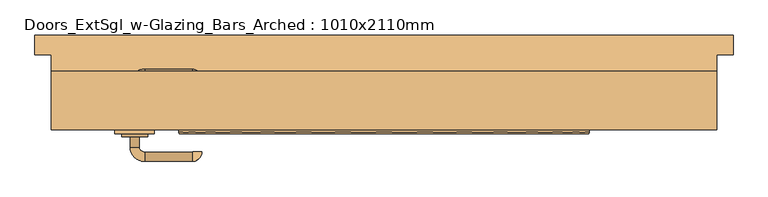
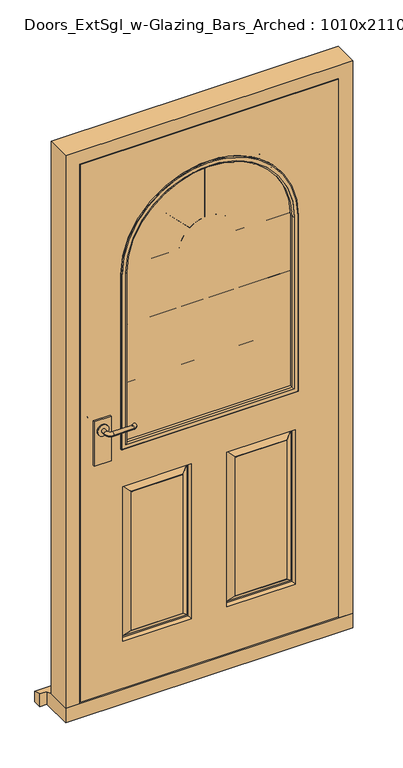
"""IFC4 building model written with IfcOpenShell, lengths in millimetres: door geometry, Doors_ExtSgl_w-Glazing_Bars_Arched : 1010x2110mm."""

from ifc_helpers import new_model, si_unit, point, frame, frame_2d, origin, place, context, project, spatial, polyline, circle_curve, ellipse_curve, trimmed, segment, composite_curve, outline, extrude, faceted_brep, source, transform, mapped, element, save
from ifc_brep_helpers import plane_surface, cylinder_surface, revolved_surface, advanced_brep


def doors_extsgl_w_glazing_bars_arched_1010x2110mm_bccdb1b2(model_context):
    return source(origin(), model_context, "Body", "SolidModel", [
        extrude(outline(composite_curve([segment(trimmed(circle_curve(frame_2d((1050.0, -378.5)), 20.0), [point((1050.0, -398.5))], [point((1050.0, -358.5))], False, "CARTESIAN"), True, "CONTINUOUS"), segment(trimmed(circle_curve(frame_2d((1050.0, -378.5)), 20.0), [point((1050.0, -358.5))], [point((1050.0, -398.5))], False, "CARTESIAN"), True, "CONTINUOUS")], self_intersect=False)), frame((0.0, -22.9929895, 0.0), z_axis=(0.0, 1.0, 0.0), x_axis=(0.0, 0.0, 1.0)), (0.0, 0.0, 1.0), 4.5929895),
        advanced_brep(
        [(-371.5, -22.9929895, 1050.0), (-385.5, -22.9929895, 1050.0), (-385.5, -38.4, 1050.0), (-371.5, -38.4, 1050.0), (-363.5, -60.4, 1050.0), (-363.5, -46.4, 1050.0), (-291.5, -60.4, 1050.0), (-291.5, -46.4, 1050.0), (-290.5, -45.4, 1050.0), (-276.5, -45.4, 1050.0)],
        [
            (0, 1, circle_curve(frame((-378.5, -22.9929895, 1050.0), z_axis=(0.0, 1.0, 0.0), x_axis=(-1.0, 0.0, 0.0)), 7.0)),
            (1, 0, circle_curve(frame((-378.5, -22.9929895, 1050.0), z_axis=(0.0, 1.0, 0.0), x_axis=(-1.0, 0.0, 0.0)), 7.0)),
            (1, 2),
            (2, 3, circle_curve(frame((-378.5, -38.4, 1050.0), z_axis=(0.0, 1.0, 0.0), x_axis=(-1.0, 0.0, 0.0)), 7.0)),
            (3, 0),
            (3, 2, circle_curve(frame((-378.5, -38.4, 1050.0), z_axis=(0.0, 1.0, 0.0), x_axis=(-1.0, 0.0, 0.0)), 7.0)),
            (4, 5, circle_curve(frame((-363.5, -53.4, 1050.0), z_axis=(-1.0, 0.0, 0.0), x_axis=(0.0, -1.0, 0.0)), 7.0)),
            (5, 3, circle_curve(frame((-363.5, -38.4, 1050.0), z_axis=(0.0, 0.0, -1.0), x_axis=(-1.0, 0.0, 0.0)), 8.0)),
            (2, 4, circle_curve(frame((-363.5, -38.4, 1050.0), z_axis=(0.0, 0.0, 1.0), x_axis=(-1.0, 0.0, 0.0)), 22.0)),
            (5, 4, circle_curve(frame((-363.5, -53.4, 1050.0), z_axis=(-1.0, 0.0, 0.0), x_axis=(0.0, -1.0, 0.0)), 7.0)),
            (4, 6),
            (6, 7, circle_curve(frame((-291.5, -53.4, 1050.0), z_axis=(-1.0, 0.0, 0.0), x_axis=(0.0, -1.0, 0.0)), 7.0)),
            (7, 5),
            (7, 6, circle_curve(frame((-291.5, -53.4, 1050.0), z_axis=(-1.0, 0.0, 0.0), x_axis=(0.0, -1.0, 0.0)), 7.0)),
            (8, 9, circle_curve(frame((-283.5, -45.4, 1050.0), z_axis=(0.0, 1.0, 0.0), x_axis=(1.0, 0.0, 0.0)), 7.0)),
            (9, 8, circle_curve(frame((-283.5, -45.4, 1050.0), z_axis=(0.0, 1.0, 0.0), x_axis=(1.0, 0.0, 0.0)), 7.0)),
            (8, 7, circle_curve(frame((-291.5, -45.4, 1050.0), z_axis=(0.0, 0.0, -1.0), x_axis=(0.0, -1.0, 0.0)), 1.0)),
            (6, 9, circle_curve(frame((-291.5, -45.4, 1050.0), z_axis=(0.0, 0.0, 1.0), x_axis=(0.0, -1.0, 0.0)), 15.0)),
        ],
        [
            plane_surface(frame((-378.5, -22.9929895, 1050.0), z_axis=(0.0, 1.0, 0.0), x_axis=(0.0, 0.0, 1.0))),
            cylinder_surface(frame((-378.5, -22.9929895, 1050.0), z_axis=(0.0, 1.0, 0.0), x_axis=(-1.0, 0.0, 0.0)), 7.0),
            revolved_surface(trimmed(ellipse_curve(frame((-378.5, -38.4, 1050.0), z_axis=(0.0, -1.0, 0.0), x_axis=(-1.0, 0.0, 0.0)), 7.0, 7.0), [point((-371.5, -38.4, 1050.0))], [point((-385.5, -38.4, 1050.0))], True, "CARTESIAN"), (-363.5, -38.4, 1050.0), (0.0, 0.0, -1.0)),
            revolved_surface(trimmed(ellipse_curve(frame((-378.5, -38.4, 1050.0), z_axis=(0.0, -1.0, 0.0), x_axis=(-1.0, 0.0, 0.0)), 7.0, 7.0), [point((-385.5, -38.4, 1050.0))], [point((-371.5, -38.4, 1050.0))], True, "CARTESIAN"), (-363.5, -38.4, 1050.0), (0.0, 0.0, -1.0)),
            cylinder_surface(frame((-363.5, -53.4, 1050.0), z_axis=(-1.0, 0.0, 0.0), x_axis=(0.0, -1.0, 0.0)), 7.0),
            plane_surface(frame((-283.5, -45.4, 1050.0), z_axis=(0.0, 1.0, 0.0), x_axis=(0.0, 0.0, 1.0))),
            revolved_surface(trimmed(ellipse_curve(frame((-291.5, -53.4, 1050.0), z_axis=(1.0, 0.0, 0.0), x_axis=(0.0, -1.0, 0.0)), 7.0, 7.0), [point((-291.5, -46.4, 1050.0))], [point((-291.5, -60.4, 1050.0))], True, "CARTESIAN"), (-291.5, -45.4, 1050.0), (0.0, 0.0, -1.0)),
            revolved_surface(trimmed(ellipse_curve(frame((-291.5, -53.4, 1050.0), z_axis=(1.0, 0.0, 0.0), x_axis=(0.0, -1.0, 0.0)), 7.0, 7.0), [point((-291.5, -60.4, 1050.0))], [point((-291.5, -46.4, 1050.0))], True, "CARTESIAN"), (-291.5, -45.4, 1050.0), (0.0, 0.0, -1.0)),
        ],
        [
            (0, [[1, 2]]),
            (1, [[3, 4, 5, -2]]),
            (1, [[-5, 6, -3, -1]]),
            (2, [[7, 8, -4, 9]]),
            (3, [[10, -9, -6, -8]]),
            (4, [[11, 12, 13, -7]]),
            (4, [[-13, 14, -11, -10]]),
            (5, [[15, 16]]),
            (6, [[-15, 17, -12, 18]]),
            (7, [[-16, -18, -14, -17]]),
        ],
    ),
        extrude(outline(polyline([(-348.5, -12.4), (-348.5, -18.4), (-408.5, -18.4), (-408.5, -12.4), (-348.5, -12.4)])), frame((0.0, 0.0, 925.0), z_axis=(0.0, 0.0, 1.0), x_axis=(1.0, 0.0, 0.0)), (0.0, 0.0, 1.0), 165.0),
        extrude(outline(composite_curve([segment(trimmed(circle_curve(frame_2d((1050.0, -378.5)), 20.0), [point((1050.0, -398.5))], [point((1050.0, -358.5))], False, "CARTESIAN"), True, "CONTINUOUS"), segment(trimmed(circle_curve(frame_2d((1050.0, -378.5)), 20.0), [point((1050.0, -358.5))], [point((1050.0, -398.5))], False, "CARTESIAN"), True, "CONTINUOUS")], self_intersect=False)), frame((0.0, 37.6, 0.0), z_axis=(0.0, 1.0, 0.0), x_axis=(0.0, 0.0, 1.0)), (0.0, 0.0, 1.0), 4.5929895),
        advanced_brep(
        [(-371.5, 42.1929895, 1050.0), (-385.5, 42.1929895, 1050.0), (-371.5, 57.6, 1050.0), (-385.5, 57.6, 1050.0), (-363.5, 79.6, 1050.0), (-363.5, 65.6, 1050.0), (-291.5, 65.6, 1050.0), (-291.5, 79.6, 1050.0), (-290.5, 64.6, 1050.0), (-276.5, 64.6, 1050.0)],
        [
            (0, 1, circle_curve(frame((-378.5, 42.1929895, 1050.0), z_axis=(0.0, -1.0, 0.0), x_axis=(-1.0, 0.0, 0.0)), 7.0)),
            (1, 0, circle_curve(frame((-378.5, 42.1929895, 1050.0), z_axis=(0.0, -1.0, 0.0), x_axis=(-1.0, 0.0, 0.0)), 7.0)),
            (0, 2),
            (2, 3, circle_curve(frame((-378.5, 57.6, 1050.0), z_axis=(0.0, -1.0, 0.0), x_axis=(-1.0, 0.0, 0.0)), 7.0)),
            (3, 1),
            (3, 2, circle_curve(frame((-378.5, 57.6, 1050.0), z_axis=(0.0, -1.0, 0.0), x_axis=(-1.0, 0.0, 0.0)), 7.0)),
            (4, 3, circle_curve(frame((-363.5, 57.6, 1050.0), z_axis=(0.0, 0.0, 1.0), x_axis=(-1.0, 0.0, 0.0)), 22.0)),
            (2, 5, circle_curve(frame((-363.5, 57.6, 1050.0), z_axis=(0.0, 0.0, -1.0), x_axis=(-1.0, 0.0, 0.0)), 8.0)),
            (5, 4, circle_curve(frame((-363.5, 72.6, 1050.0), z_axis=(-1.0, 0.0, 0.0), x_axis=(0.0, 1.0, 0.0)), 7.0)),
            (4, 5, circle_curve(frame((-363.5, 72.6, 1050.0), z_axis=(-1.0, 0.0, 0.0), x_axis=(0.0, 1.0, 0.0)), 7.0)),
            (5, 6),
            (6, 7, circle_curve(frame((-291.5, 72.6, 1050.0), z_axis=(-1.0, 0.0, 0.0), x_axis=(0.0, 1.0, 0.0)), 7.0)),
            (7, 4),
            (7, 6, circle_curve(frame((-291.5, 72.6, 1050.0), z_axis=(-1.0, 0.0, 0.0), x_axis=(0.0, 1.0, 0.0)), 7.0)),
            (8, 9, circle_curve(frame((-283.5, 64.6, 1050.0), z_axis=(0.0, -1.0, 0.0), x_axis=(1.0, 0.0, 0.0)), 7.0)),
            (9, 8, circle_curve(frame((-283.5, 64.6, 1050.0), z_axis=(0.0, -1.0, 0.0), x_axis=(1.0, 0.0, 0.0)), 7.0)),
            (9, 7, circle_curve(frame((-291.5, 64.6, 1050.0), z_axis=(0.0, 0.0, 1.0), x_axis=(0.0, 1.0, 0.0)), 15.0)),
            (6, 8, circle_curve(frame((-291.5, 64.6, 1050.0), z_axis=(0.0, 0.0, -1.0), x_axis=(0.0, 1.0, 0.0)), 1.0)),
        ],
        [
            plane_surface(frame((-378.5, 42.1929895, 1050.0), z_axis=(0.0, -1.0, 0.0), x_axis=(0.0, 0.0, 1.0))),
            cylinder_surface(frame((-378.5, 42.1929895, 1050.0), z_axis=(0.0, -1.0, 0.0), x_axis=(-1.0, 0.0, 0.0)), 7.0),
            revolved_surface(trimmed(ellipse_curve(frame((-378.5, 57.6, 1050.0), z_axis=(0.0, -1.0, 0.0), x_axis=(-1.0, 0.0, 0.0)), 7.0, 7.0), [point((-371.5, 57.6, 1050.0))], [point((-385.5, 57.6, 1050.0))], True, "CARTESIAN"), (-363.5, 57.6, 1050.0), (0.0, 0.0, -1.0)),
            revolved_surface(trimmed(ellipse_curve(frame((-378.5, 57.6, 1050.0), z_axis=(0.0, -1.0, 0.0), x_axis=(-1.0, 0.0, 0.0)), 7.0, 7.0), [point((-385.5, 57.6, 1050.0))], [point((-371.5, 57.6, 1050.0))], True, "CARTESIAN"), (-363.5, 57.6, 1050.0), (0.0, 0.0, -1.0)),
            cylinder_surface(frame((-363.5, 72.6, 1050.0), z_axis=(-1.0, 0.0, 0.0), x_axis=(0.0, 1.0, 0.0)), 7.0),
            plane_surface(frame((-283.5, 64.6, 1050.0), z_axis=(0.0, -1.0, 0.0), x_axis=(0.0, 0.0, 1.0))),
            revolved_surface(trimmed(ellipse_curve(frame((-291.5, 72.6, 1050.0), z_axis=(-1.0, 0.0, 0.0), x_axis=(0.0, 1.0, 0.0)), 7.0, 7.0), [point((-291.5, 65.6, 1050.0))], [point((-291.5, 79.6, 1050.0))], True, "CARTESIAN"), (-291.5, 64.6, 1050.0), (0.0, 0.0, -1.0)),
            revolved_surface(trimmed(ellipse_curve(frame((-291.5, 72.6, 1050.0), z_axis=(-1.0, 0.0, 0.0), x_axis=(0.0, 1.0, 0.0)), 7.0, 7.0), [point((-291.5, 79.6, 1050.0))], [point((-291.5, 65.6, 1050.0))], True, "CARTESIAN"), (-291.5, 64.6, 1050.0), (0.0, 0.0, -1.0)),
        ],
        [
            (0, [[1, 2]]),
            (1, [[-1, 3, 4, 5]]),
            (1, [[-2, -5, 6, -3]]),
            (2, [[7, -4, 8, 9]]),
            (3, [[-8, -6, -7, 10]]),
            (4, [[-9, 11, 12, 13]]),
            (4, [[-10, -13, 14, -11]]),
            (5, [[15, 16]]),
            (6, [[17, -12, 18, -16]]),
            (7, [[-18, -14, -17, -15]]),
        ],
    ),
        extrude(outline(polyline([(-348.5, 31.6), (-408.5, 31.6), (-408.5, 37.6), (-348.5, 37.6), (-348.5, 31.6)])), frame((0.0, 0.0, 925.0), z_axis=(0.0, 0.0, 1.0), x_axis=(1.0, 0.0, 0.0)), (0.0, 0.0, 1.0), 165.0),
        faceted_brep([(434.5, 76.6, 54.5), (505.0, 76.6, 54.5), (505.0, -12.4, 54.5), (456.5, -12.4, 54.5), (456.5, 34.6, 54.5), (434.5, 34.6, 54.5), (434.5, 76.6, 2039.5), (-434.5, 76.6, 2039.5), (-434.5, 76.6, 54.5), (-505.0, 76.6, 54.5), (-505.0, 76.6, 2110.0), (505.0, 76.6, 2110.0), (505.0, -12.4, 2110.0), (-505.0, -12.4, 2110.0), (-505.0, -12.4, 54.5), (-456.5, -12.4, 54.5), (-456.5, -12.4, 2061.5), (456.5, -12.4, 2061.5), (456.5, 34.6, 2061.5), (-456.5, 34.6, 2061.5), (-456.5, 34.6, 54.5), (-434.5, 34.6, 54.5), (-434.5, 34.6, 2039.5), (434.5, 34.6, 2039.5)], [[[0, 1, 2, 3, 4, 5]], [[1, 0, 6, 7, 8, 9, 10, 11]], [[2, 1, 11, 12]], [[3, 2, 12, 13, 14, 15, 16, 17]], [[4, 3, 17, 18]], [[5, 4, 18, 19, 20, 21, 22, 23]], [[0, 5, 23, 6]], [[8, 7, 22, 21]], [[9, 8, 21, 20, 15, 14]], [[10, 9, 14, 13]], [[16, 15, 20, 19]], [[11, 10, 13, 12]], [[17, 16, 19, 18]], [[7, 6, 23, 22]]]),
        advanced_brep(
        [(453.5, -12.4, 58.5), (453.5, -12.4, 2058.5), (-454.4250294, -12.4, 2058.5), (-454.4250294, -12.4, 58.5), (-303.5, -12.4, 958.5), (-303.5, -12.4, 1605.0), (303.5, -12.4, 1605.0), (303.5, -12.4, 958.5), (-62.5, -12.4, 808.5), (-62.5, -12.4, 233.5), (-303.5, -12.4, 233.5), (-303.5, -12.4, 808.5), (303.5, -12.4, 808.5), (303.5, -12.4, 233.5), (62.5, -12.4, 233.5), (62.5, -12.4, 808.5), (-92.5, -12.4, 263.5), (-92.5, -12.4, 778.5), (-273.5, -12.4, 778.5), (-273.5, -12.4, 263.5), (273.5, -12.4, 263.5), (273.5, -12.4, 778.5), (92.5, -12.4, 778.5), (92.5, -12.4, 263.5), (453.5, 31.6, 58.5), (-454.4250294, 31.6, 58.5), (-454.4250294, 31.6, 2058.5), (453.5, 31.6, 2058.5), (-303.5, 31.6, 958.5), (303.5, 31.6, 958.5), (303.5, 31.6, 1605.0), (-303.5, 31.6, 1605.0), (62.5, 31.6, 808.5), (62.5, 31.6, 233.5), (303.5, 31.6, 233.5), (303.5, 31.6, 808.5), (-303.5, 31.6, 808.5), (-303.5, 31.6, 233.5), (-62.5, 31.6, 233.5), (-62.5, 31.6, 808.5), (92.5, 31.6, 263.5), (92.5, 31.6, 778.5), (273.5, 31.6, 778.5), (273.5, 31.6, 263.5), (-273.5, 31.6, 263.5), (-273.5, 31.6, 778.5), (-92.5, 31.6, 778.5), (-92.5, 31.6, 263.5), (65.5, 16.6, 805.5), (65.5, 16.6, 236.5), (90.5, 30.6, 780.5), (90.5, 30.6, 261.5), (70.5, 16.6, 241.5), (70.5, 16.6, 800.5), (92.5, 30.6, 263.5), (92.5, 30.6, 778.5), (300.5, 16.6, 236.5), (275.5, 30.6, 261.5), (295.5, 16.6, 241.5), (273.5, 30.6, 263.5), (300.5, 16.6, 805.5), (275.5, 30.6, 780.5), (295.5, 16.6, 800.5), (273.5, 30.6, 778.5), (-300.5, 16.6, 805.5), (-300.5, 16.6, 236.5), (-275.5, 30.6, 780.5), (-275.5, 30.6, 261.5), (-295.5, 16.6, 241.5), (-295.5, 16.6, 800.5), (-273.5, 30.6, 263.5), (-273.5, 30.6, 778.5), (-65.5, 16.6, 236.5), (-90.5, 30.6, 261.5), (-70.5, 16.6, 241.5), (-92.5, 30.6, 263.5), (-65.5, 16.6, 805.5), (-90.5, 30.6, 780.5), (-70.5, 16.6, 800.5), (-92.5, 30.6, 778.5), (-92.5, -11.4, 263.5), (-92.5, -11.4, 778.5), (-70.5, 2.6, 241.5), (-70.5, 2.6, 800.5), (-90.5, -11.4, 780.5), (-90.5, -11.4, 261.5), (-65.5, 2.6, 805.5), (-65.5, 2.6, 236.5), (-273.5, -11.4, 778.5), (-295.5, 2.6, 800.5), (-275.5, -11.4, 780.5), (-300.5, 2.6, 805.5), (-273.5, -11.4, 263.5), (-295.5, 2.6, 241.5), (-275.5, -11.4, 261.5), (-300.5, 2.6, 236.5), (300.5, 2.6, 805.5), (300.5, 2.6, 236.5), (275.5, -11.4, 780.5), (275.5, -11.4, 261.5), (295.5, 2.6, 241.5), (295.5, 2.6, 800.5), (273.5, -11.4, 263.5), (273.5, -11.4, 778.5), (65.5, 2.6, 236.5), (90.5, -11.4, 261.5), (70.5, 2.6, 241.5), (92.5, -11.4, 263.5), (65.5, 2.6, 805.5), (90.5, -11.4, 780.5), (70.5, 2.6, 800.5), (92.5, -11.4, 778.5)],
        [
            (0, 1),
            (1, 2),
            (2, 3),
            (3, 0),
            (4, 5),
            (5, 6, circle_curve(frame((0.0, -12.4, 1605.0), z_axis=(0.0, 1.0, 0.0), x_axis=(1.0, 0.0, 0.0)), 303.5)),
            (6, 7),
            (7, 4),
            (8, 9),
            (9, 10),
            (10, 11),
            (11, 8),
            (12, 13),
            (13, 14),
            (14, 15),
            (15, 12),
            (16, 17),
            (17, 18),
            (18, 19),
            (19, 16),
            (20, 21),
            (21, 22),
            (22, 23),
            (23, 20),
            (24, 25),
            (25, 26),
            (26, 27),
            (27, 24),
            (28, 29),
            (29, 30),
            (30, 31, circle_curve(frame((0.0, 31.6, 1605.0), z_axis=(0.0, -1.0, 0.0), x_axis=(1.0, 0.0, 0.0)), 303.5)),
            (31, 28),
            (32, 33),
            (33, 34),
            (34, 35),
            (35, 32),
            (36, 37),
            (37, 38),
            (38, 39),
            (39, 36),
            (40, 41),
            (41, 42),
            (42, 43),
            (43, 40),
            (44, 45),
            (45, 46),
            (46, 47),
            (47, 44),
            (0, 24),
            (27, 1),
            (26, 2),
            (25, 3),
            (4, 28),
            (31, 5),
            (30, 6),
            (29, 7),
            (48, 49),
            (49, 33),
            (32, 48),
            (50, 51),
            (51, 52),
            (52, 53),
            (53, 50),
            (40, 54),
            (54, 55),
            (55, 41),
            (49, 56),
            (56, 34),
            (51, 57),
            (57, 58),
            (58, 52),
            (43, 59),
            (59, 54),
            (56, 60),
            (60, 35),
            (57, 61),
            (61, 62),
            (62, 58),
            (42, 63),
            (63, 59),
            (60, 48),
            (62, 53),
            (61, 50),
            (63, 55),
            (64, 65),
            (65, 37),
            (36, 64),
            (66, 67),
            (67, 68),
            (68, 69),
            (69, 66),
            (44, 70),
            (70, 71),
            (71, 45),
            (65, 72),
            (72, 38),
            (67, 73),
            (73, 74),
            (74, 68),
            (47, 75),
            (75, 70),
            (72, 76),
            (76, 39),
            (73, 77),
            (77, 78),
            (78, 74),
            (46, 79),
            (79, 75),
            (76, 64),
            (78, 69),
            (77, 66),
            (79, 71),
            (80, 81),
            (81, 17),
            (16, 80),
            (82, 83),
            (83, 84),
            (84, 85),
            (85, 82),
            (8, 86),
            (86, 87),
            (87, 9),
            (81, 88),
            (88, 18),
            (83, 89),
            (89, 90),
            (90, 84),
            (11, 91),
            (91, 86),
            (88, 92),
            (92, 19),
            (89, 93),
            (93, 94),
            (94, 90),
            (10, 95),
            (95, 91),
            (92, 80),
            (94, 85),
            (93, 82),
            (95, 87),
            (96, 97),
            (97, 13),
            (12, 96),
            (98, 99),
            (99, 100),
            (100, 101),
            (101, 98),
            (20, 102),
            (102, 103),
            (103, 21),
            (97, 104),
            (104, 14),
            (99, 105),
            (105, 106),
            (106, 100),
            (23, 107),
            (107, 102),
            (104, 108),
            (108, 15),
            (105, 109),
            (109, 110),
            (110, 106),
            (22, 111),
            (111, 107),
            (108, 96),
            (110, 101),
            (109, 98),
            (111, 103),
        ],
        [
            plane_surface(frame((453.5, -12.4, 58.5), z_axis=(0.0, -1.0, 0.0), x_axis=(0.0, 0.0, 1.0))),
            plane_surface(frame((453.5, 31.6, 58.5), z_axis=(0.0, 1.0, 0.0), x_axis=(0.0, 0.0, -1.0))),
            plane_surface(frame((453.5, -12.4, 58.5), z_axis=(1.0, 0.0, 0.0), x_axis=(0.0, 1.0, 0.0))),
            plane_surface(frame((453.5, -12.4, 2058.5), z_axis=(0.0, 0.0, 1.0), x_axis=(0.0, 1.0, 0.0))),
            plane_surface(frame((-454.4250294, -12.4, 2058.5), z_axis=(-1.0, 0.0, 0.0), x_axis=(0.0, 1.0, 0.0))),
            plane_surface(frame((-454.4250294, -12.4, 58.5), z_axis=(0.0, 0.0, -1.0), x_axis=(0.0, 1.0, 0.0))),
            plane_surface(frame((-303.5, -12.4, 958.5), z_axis=(1.0, 0.0, 0.0), x_axis=(0.0, 1.0, 0.0))),
            revolved_surface(polyline([(303.5, 31.6, 1605.0), (303.5, -12.4, 1605.0)]), (0.0, -12.4, 1605.0), (0.0, 1.0, 0.0)),
            plane_surface(frame((303.5, -12.4, 1605.0), z_axis=(-1.0, 0.0, 0.0), x_axis=(0.0, 1.0, 0.0))),
            plane_surface(frame((303.5, -12.4, 958.5), z_axis=(0.0, 0.0, 1.0), x_axis=(0.0, 1.0, 0.0))),
            plane_surface(frame((62.5, 31.6, 808.5), z_axis=(0.9805806756909202, 0.19611613513818407, 0.0), x_axis=(0.0, 0.0, -1.0))),
            plane_surface(frame((70.5, 16.6, 800.5), z_axis=(-0.5734623443633278, 0.8192319205190408, 0.0), x_axis=(0.0, 0.0, -1.0))),
            plane_surface(frame((92.5, 30.6, 778.5), z_axis=(-1.0, 0.0, 0.0), x_axis=(0.0, 0.0, -1.0))),
            plane_surface(frame((62.5, 31.6, 233.5), z_axis=(0.0, 0.19611613513818726, 0.9805806756909196), x_axis=(1.0, 0.0, 0.0))),
            plane_surface(frame((70.5, 16.6, 241.5), z_axis=(0.0, 0.819231920519039, -0.5734623443633305), x_axis=(1.0, 0.0, 0.0))),
            plane_surface(frame((92.5, 30.6, 263.5), z_axis=(0.0, 0.0, -1.0), x_axis=(1.0, 0.0, 0.0))),
            plane_surface(frame((303.5, 31.6, 233.5), z_axis=(-0.9805806756909189, 0.19611613513819046, 0.0), x_axis=(0.0, 0.0, 1.0))),
            plane_surface(frame((295.5, 16.6, 241.5), z_axis=(0.5734623443633332, 0.8192319205190371, 0.0), x_axis=(0.0, 0.0, 1.0))),
            plane_surface(frame((273.5, 30.6, 263.5), z_axis=(1.0, 0.0, 0.0), x_axis=(0.0, 0.0, 1.0))),
            plane_surface(frame((303.5, 31.6, 808.5), z_axis=(0.0, 0.19611613513818726, -0.9805806756909196), x_axis=(-1.0, 0.0, 0.0))),
            plane_surface(frame((300.5, 16.6, 805.5), z_axis=(0.0, 1.0, 0.0), x_axis=(-1.0, 0.0, 0.0))),
            plane_surface(frame((295.5, 16.6, 800.5), z_axis=(0.0, 0.819231920519039, 0.5734623443633305), x_axis=(-1.0, 0.0, 0.0))),
            plane_surface(frame((275.5, 30.6, 780.5), z_axis=(0.0, 1.0, 0.0), x_axis=(-1.0, 0.0, 0.0))),
            plane_surface(frame((273.5, 30.6, 778.5), z_axis=(0.0, 0.0, 1.0), x_axis=(-1.0, 0.0, 0.0))),
            plane_surface(frame((-303.5, 31.6, 808.5), z_axis=(0.9805806756909202, 0.19611613513818407, 0.0), x_axis=(0.0, 0.0, -1.0))),
            plane_surface(frame((-295.5, 16.6, 800.5), z_axis=(-0.5734623443633278, 0.8192319205190408, 0.0), x_axis=(0.0, 0.0, -1.0))),
            plane_surface(frame((-273.5, 30.6, 778.5), z_axis=(-1.0, 0.0, 0.0), x_axis=(0.0, 0.0, -1.0))),
            plane_surface(frame((-303.5, 31.6, 233.5), z_axis=(0.0, 0.19611613513818724, 0.9805806756909196), x_axis=(1.0, 0.0, 0.0))),
            plane_surface(frame((-295.5, 16.6, 241.5), z_axis=(0.0, 0.819231920519039, -0.5734623443633305), x_axis=(1.0, 0.0, 0.0))),
            plane_surface(frame((-273.5, 30.6, 263.5), z_axis=(0.0, 0.0, -1.0), x_axis=(1.0, 0.0, 0.0))),
            plane_surface(frame((-62.5, 31.6, 233.5), z_axis=(-0.9805806756909189, 0.1961161351381904, 0.0), x_axis=(0.0, 0.0, 1.0))),
            plane_surface(frame((-70.5, 16.6, 241.5), z_axis=(0.5734623443633332, 0.8192319205190371, 0.0), x_axis=(0.0, 0.0, 1.0))),
            plane_surface(frame((-92.5, 30.6, 263.5), z_axis=(1.0, 0.0, 0.0), x_axis=(0.0, 0.0, 1.0))),
            plane_surface(frame((-62.5, 31.6, 808.5), z_axis=(0.0, 0.19611613513818724, -0.9805806756909196), x_axis=(-1.0, 0.0, 0.0))),
            plane_surface(frame((-65.5, 16.6, 805.5), z_axis=(0.0, 1.0, 0.0), x_axis=(-1.0, 0.0, 0.0))),
            plane_surface(frame((-70.5, 16.6, 800.5), z_axis=(0.0, 0.819231920519039, 0.5734623443633305), x_axis=(-1.0, 0.0, 0.0))),
            plane_surface(frame((-90.5, 30.6, 780.5), z_axis=(0.0, 1.0, 0.0), x_axis=(-1.0, 0.0, 0.0))),
            plane_surface(frame((-92.5, 30.6, 778.5), z_axis=(0.0, 0.0, 1.0), x_axis=(-1.0, 0.0, 0.0))),
            plane_surface(frame((-92.5, -12.4, 263.5), z_axis=(1.0, 0.0, 0.0), x_axis=(0.0, 0.0, 1.0))),
            plane_surface(frame((-90.5, -11.4, 261.5), z_axis=(0.5734623443633224, -0.8192319205190447, 0.0), x_axis=(0.0, 0.0, 1.0))),
            plane_surface(frame((-65.5, 2.6, 236.5), z_axis=(-0.9805806756909214, -0.1961161351381778, 0.0), x_axis=(0.0, 0.0, 1.0))),
            plane_surface(frame((-92.5, -12.4, 778.5), z_axis=(0.0, 0.0, 1.0), x_axis=(-1.0, 0.0, 0.0))),
            plane_surface(frame((-90.5, -11.4, 780.5), z_axis=(0.0, -0.8192319205190428, 0.5734623443633251), x_axis=(-1.0, 0.0, 0.0))),
            plane_surface(frame((-65.5, 2.6, 805.5), z_axis=(0.0, -0.19611613513818096, -0.9805806756909208), x_axis=(-1.0, 0.0, 0.0))),
            plane_surface(frame((-273.5, -12.4, 778.5), z_axis=(-1.0, 0.0, 0.0), x_axis=(0.0, 0.0, -1.0))),
            plane_surface(frame((-275.5, -11.4, 780.5), z_axis=(-0.5734623443633277, -0.8192319205190409, 0.0), x_axis=(0.0, 0.0, -1.0))),
            plane_surface(frame((-300.5, 2.6, 805.5), z_axis=(0.9805806756909201, -0.19611613513818418, 0.0), x_axis=(0.0, 0.0, -1.0))),
            plane_surface(frame((-273.5, -12.4, 263.5), z_axis=(0.0, 0.0, -1.0), x_axis=(1.0, 0.0, 0.0))),
            plane_surface(frame((-273.5, -11.4, 263.5), z_axis=(0.0, -1.0, 0.0), x_axis=(1.0, 0.0, 0.0))),
            plane_surface(frame((-275.5, -11.4, 261.5), z_axis=(0.0, -0.8192319205190429, -0.573462344363325), x_axis=(1.0, 0.0, 0.0))),
            plane_surface(frame((-295.5, 2.6, 241.5), z_axis=(0.0, -1.0, 0.0), x_axis=(1.0, 0.0, 0.0))),
            plane_surface(frame((-300.5, 2.6, 236.5), z_axis=(0.0, -0.19611613513818107, 0.9805806756909208), x_axis=(1.0, 0.0, 0.0))),
            plane_surface(frame((303.5, -12.4, 808.5), z_axis=(-0.9805806756909202, -0.19611613513818407, 0.0), x_axis=(0.0, 0.0, -1.0))),
            plane_surface(frame((295.5, 2.6, 800.5), z_axis=(0.5734623443633278, -0.8192319205190408, 0.0), x_axis=(0.0, 0.0, -1.0))),
            plane_surface(frame((273.5, -11.4, 778.5), z_axis=(1.0, 0.0, 0.0), x_axis=(0.0, 0.0, -1.0))),
            plane_surface(frame((303.5, -12.4, 233.5), z_axis=(0.0, -0.19611613513818724, 0.9805806756909196), x_axis=(-1.0, 0.0, 0.0))),
            plane_surface(frame((295.5, 2.6, 241.5), z_axis=(0.0, -0.819231920519039, -0.5734623443633305), x_axis=(-1.0, 0.0, 0.0))),
            plane_surface(frame((273.5, -11.4, 263.5), z_axis=(0.0, 0.0, -1.0), x_axis=(-1.0, 0.0, 0.0))),
            plane_surface(frame((62.5, -12.4, 233.5), z_axis=(0.9805806756909189, -0.19611613513819046, 0.0), x_axis=(0.0, 0.0, 1.0))),
            plane_surface(frame((70.5, 2.6, 241.5), z_axis=(-0.5734623443633331, -0.8192319205190371, 0.0), x_axis=(0.0, 0.0, 1.0))),
            plane_surface(frame((92.5, -11.4, 263.5), z_axis=(-1.0, 0.0, 0.0), x_axis=(0.0, 0.0, 1.0))),
            plane_surface(frame((62.5, -12.4, 808.5), z_axis=(0.0, -0.19611613513818735, -0.9805806756909196), x_axis=(1.0, 0.0, 0.0))),
            plane_surface(frame((65.5, 2.6, 805.5), z_axis=(0.0, -1.0, 0.0), x_axis=(1.0, 0.0, 0.0))),
            plane_surface(frame((70.5, 2.6, 800.5), z_axis=(0.0, -0.819231920519039, 0.5734623443633303), x_axis=(1.0, 0.0, 0.0))),
            plane_surface(frame((90.5, -11.4, 780.5), z_axis=(0.0, -1.0, 0.0), x_axis=(1.0, 0.0, 0.0))),
            plane_surface(frame((92.5, -11.4, 778.5), z_axis=(0.0, 0.0, 1.0), x_axis=(1.0, 0.0, 0.0))),
        ],
        [
            (0, [[1, 2, 3, 4], [5, 6, 7, 8], [9, 10, 11, 12], [13, 14, 15, 16]]),
            (0, [[17, 18, 19, 20]]),
            (0, [[21, 22, 23, 24]]),
            (1, [[25, 26, 27, 28], [29, 30, 31, 32], [33, 34, 35, 36], [37, 38, 39, 40]]),
            (1, [[41, 42, 43, 44]]),
            (1, [[45, 46, 47, 48]]),
            (2, [[-1, 49, -28, 50]]),
            (3, [[-2, -50, -27, 51]]),
            (4, [[-3, -51, -26, 52]]),
            (5, [[-4, -52, -25, -49]]),
            (6, [[-5, 53, -32, 54]]),
            (7, [[-6, -54, -31, 55]]),
            (8, [[-7, -55, -30, 56]]),
            (9, [[-8, -56, -29, -53]]),
            (10, [[57, 58, -33, 59]]),
            (11, [[60, 61, 62, 63]]),
            (12, [[64, 65, 66, -41]]),
            (13, [[-58, 67, 68, -34]]),
            (14, [[-61, 69, 70, 71]]),
            (15, [[-64, -44, 72, 73]]),
            (16, [[-68, 74, 75, -35]]),
            (17, [[-70, 76, 77, 78]]),
            (18, [[-72, -43, 79, 80]]),
            (19, [[-59, -36, -75, 81]]),
            (20, [[-57, -81, -74, -67], [-62, -71, -78, 82]]),
            (21, [[-63, -82, -77, 83]]),
            (22, [[-60, -83, -76, -69], [-65, -73, -80, 84]]),
            (23, [[-66, -84, -79, -42]]),
            (24, [[85, 86, -37, 87]]),
            (25, [[88, 89, 90, 91]]),
            (26, [[92, 93, 94, -45]]),
            (27, [[-86, 95, 96, -38]]),
            (28, [[-89, 97, 98, 99]]),
            (29, [[-92, -48, 100, 101]]),
            (30, [[-96, 102, 103, -39]]),
            (31, [[-98, 104, 105, 106]]),
            (32, [[-100, -47, 107, 108]]),
            (33, [[-87, -40, -103, 109]]),
            (34, [[-85, -109, -102, -95], [-90, -99, -106, 110]]),
            (35, [[-91, -110, -105, 111]]),
            (36, [[-88, -111, -104, -97], [-93, -101, -108, 112]]),
            (37, [[-94, -112, -107, -46]]),
            (38, [[113, 114, -17, 115]]),
            (39, [[116, 117, 118, 119]]),
            (40, [[120, 121, 122, -9]]),
            (41, [[-114, 123, 124, -18]]),
            (42, [[-117, 125, 126, 127]]),
            (43, [[-120, -12, 128, 129]]),
            (44, [[-124, 130, 131, -19]]),
            (45, [[-126, 132, 133, 134]]),
            (46, [[-128, -11, 135, 136]]),
            (47, [[-115, -20, -131, 137]]),
            (48, [[-118, -127, -134, 138], [-113, -137, -130, -123]]),
            (49, [[-119, -138, -133, 139]]),
            (50, [[-121, -129, -136, 140], [-116, -139, -132, -125]]),
            (51, [[-122, -140, -135, -10]]),
            (52, [[141, 142, -13, 143]]),
            (53, [[144, 145, 146, 147]]),
            (54, [[148, 149, 150, -21]]),
            (55, [[-142, 151, 152, -14]]),
            (56, [[-145, 153, 154, 155]]),
            (57, [[-148, -24, 156, 157]]),
            (58, [[-152, 158, 159, -15]]),
            (59, [[-154, 160, 161, 162]]),
            (60, [[-156, -23, 163, 164]]),
            (61, [[-143, -16, -159, 165]]),
            (62, [[-141, -165, -158, -151], [-146, -155, -162, 166]]),
            (63, [[-147, -166, -161, 167]]),
            (64, [[-144, -167, -160, -153], [-149, -157, -164, 168]]),
            (65, [[-150, -168, -163, -22]]),
        ],
    ),
        faceted_brep([(530.0, 131.6, 0.0), (530.0, 131.6, 38.5947221), (530.0, 101.6, 47.2703282), (530.0, 101.6, 0.0), (-530.0, 131.6, 38.5947221), (-530.0, 131.6, 0.0), (-530.0, 101.6, 0.0), (-530.0, 101.6, 47.2703282), (505.0, 101.6, 0.0), (505.0, -12.4, 0.0), (-505.0, -12.4, 0.0), (-505.0, 101.6, 0.0), (-505.0, 101.6, 47.2703282), (-505.0, 76.6, 54.5), (505.0, 76.6, 54.5), (505.0, 101.6, 47.2703282), (-505.0, -12.4, 54.5), (505.0, -12.4, 54.5)], [[[0, 1, 2, 3]], [[4, 5, 6, 7]], [[5, 0, 3, 8, 9, 10, 11, 6]], [[1, 0, 5, 4]], [[1, 4, 7, 12, 13, 14, 15, 2]], [[13, 16, 17, 14]], [[16, 10, 9, 17]], [[12, 11, 10, 16, 13]], [[11, 12, 7, 6]], [[8, 15, 14, 17, 9]], [[15, 8, 3, 2]]]),
        extrude(outline(composite_curve([segment(polyline([(958.5, -303.5), (958.5, 303.5), (1605.0, 303.5)]), True, "CONTINUOUS"), segment(trimmed(circle_curve(frame_2d((1605.0, 0.0)), 303.5), [point((1605.0, 303.5))], [point((1605.0, -303.5))], False, "CARTESIAN"), True, "CONTINUOUS"), segment(polyline([(1605.0, -303.5), (958.5, -303.5)]), True, "CONTINUOUS")], self_intersect=False)), frame((0.0, -2.4, 0.0), z_axis=(0.0, 1.0, 0.0), x_axis=(0.0, 0.0, 1.0)), (0.0, 0.0, 1.0), 24.0),
        advanced_brep(
        [(-311.5, 35.6, 950.5), (-311.5, 31.6, 950.5), (-311.5, 31.6, 1605.0), (-311.5, 35.6, 1605.0), (-309.5, 37.6, 952.5), (-309.5, 37.6, 1605.0), (-291.5, 32.6, 970.5), (-296.5, 37.6, 965.5), (-296.5, 37.6, 1605.0), (-291.5, 32.6, 1605.0), (-291.5, 21.6, 970.5), (-291.5, 21.6, 1605.0), (-303.5, 31.6, 958.5), (-303.5, 21.6, 958.5), (-303.5, 21.6, 1605.0), (-303.5, 31.6, 1605.0), (311.5, 35.6, 1605.0), (311.5, 31.6, 1605.0), (309.5, 37.6, 1605.0), (309.5, 37.6, 952.5), (296.5, 37.6, 1605.0), (296.5, 37.6, 965.5), (291.5, 32.6, 1605.0), (291.5, 21.6, 1605.0), (303.5, 21.6, 1605.0), (303.5, 21.6, 958.5), (291.5, 21.6, 970.5), (303.5, 31.6, 1605.0), (311.5, 31.6, 950.5), (303.5, 31.6, 958.5), (311.5, 35.6, 950.5), (291.5, 32.6, 970.5)],
        [
            (0, 1),
            (1, 2),
            (2, 3),
            (3, 0),
            (4, 0, ellipse_curve(frame((-309.5, 35.6, 952.5), z_axis=(-0.7071067811865475, 0.0, 0.7071067811865475), x_axis=(-0.7071067811865472, 0.0, -0.7071067811865477)), 2.8284271, 2.0)),
            (3, 5, circle_curve(frame((-309.5, 35.6, 1605.0), z_axis=(0.0, 0.0, -1.0), x_axis=(-1.0, 0.0, 0.0)), 2.0)),
            (5, 4),
            (6, 7, ellipse_curve(frame((-296.5, 32.6, 965.5), z_axis=(-0.7071067811865475, 0.0, 0.7071067811865475), x_axis=(-0.7071067811865472, 0.0, -0.7071067811865477)), 7.0710678, 5.0)),
            (7, 8),
            (8, 9, circle_curve(frame((-296.5, 32.6, 1605.0), z_axis=(0.0, 0.0, -1.0), x_axis=(-1.0, 0.0, 0.0)), 5.0)),
            (9, 6),
            (10, 6),
            (9, 11),
            (11, 10),
            (12, 13),
            (13, 14),
            (14, 15),
            (15, 12),
            (16, 3, circle_curve(frame((0.0, 35.6, 1605.0), z_axis=(0.0, -1.0, 0.0), x_axis=(-1.0, 0.0, 0.0)), 311.5)),
            (2, 17, circle_curve(frame((0.0, 31.6, 1605.0), z_axis=(0.0, 1.0, 0.0), x_axis=(-1.0, 0.0, 0.0)), 311.5)),
            (17, 16),
            (18, 5, circle_curve(frame((0.0, 37.6, 1605.0), z_axis=(0.0, -1.0, 0.0), x_axis=(-1.0, 0.0, 0.0)), 309.5)),
            (16, 18, circle_curve(frame((309.5, 35.6, 1605.0), z_axis=(0.0, 0.0, 1.0), x_axis=(1.0, 0.0, 0.0)), 2.0)),
            (18, 19),
            (19, 4),
            (20, 8, circle_curve(frame((0.0, 37.6, 1605.0), z_axis=(0.0, -1.0, 0.0), x_axis=(-1.0, 0.0, 0.0)), 296.5)),
            (7, 21),
            (21, 20),
            (22, 9, circle_curve(frame((0.0, 32.6, 1605.0), z_axis=(0.0, -1.0, 0.0), x_axis=(-1.0, 0.0, 0.0)), 291.5)),
            (20, 22, circle_curve(frame((296.5, 32.6, 1605.0), z_axis=(0.0, 0.0, 1.0), x_axis=(1.0, 0.0, 0.0)), 5.0)),
            (23, 11, circle_curve(frame((0.0, 21.6, 1605.0), z_axis=(0.0, -1.0, 0.0), x_axis=(-1.0, 0.0, 0.0)), 291.5)),
            (22, 23),
            (24, 14, circle_curve(frame((0.0, 21.6, 1605.0), z_axis=(0.0, -1.0, 0.0), x_axis=(-1.0, 0.0, 0.0)), 303.5)),
            (13, 25),
            (25, 24),
            (23, 26),
            (26, 10),
            (27, 15, circle_curve(frame((0.0, 31.6, 1605.0), z_axis=(0.0, -1.0, 0.0), x_axis=(-1.0, 0.0, 0.0)), 303.5)),
            (24, 27),
            (1, 28),
            (28, 17),
            (27, 29),
            (29, 12),
            (28, 30),
            (30, 16),
            (30, 19, ellipse_curve(frame((309.5, 35.6, 952.5), z_axis=(0.7071067811865475, 0.0, 0.7071067811865475), x_axis=(-0.7071067811865475, 0.0, 0.7071067811865476)), 2.8284271, 2.0)),
            (21, 31, ellipse_curve(frame((296.5, 32.6, 965.5), z_axis=(0.7071067811865475, 0.0, 0.7071067811865475), x_axis=(-0.7071067811865475, 0.0, 0.7071067811865476)), 7.0710678, 5.0)),
            (31, 22),
            (31, 26),
            (25, 29),
            (0, 30),
            (6, 31),
        ],
        [
            plane_surface(frame((-311.5, 31.6, 950.5), z_axis=(-1.0, 0.0, 0.0), x_axis=(0.0, 0.0, 1.0))),
            cylinder_surface(frame((-309.5, 35.6, 958.5), z_axis=(0.0, 0.0, -1.0), x_axis=(-1.0, 0.0, 0.0)), 2.0),
            cylinder_surface(frame((-296.5, 32.6, 958.5), z_axis=(0.0, 0.0, -1.0), x_axis=(-1.0, 0.0, 0.0)), 5.0),
            plane_surface(frame((-291.5, 32.6, 970.5), z_axis=(1.0, 0.0, 0.0), x_axis=(0.0, 0.0, 1.0))),
            plane_surface(frame((-303.5, 21.6, 958.5), z_axis=(-1.0, 0.0, 0.0), x_axis=(0.0, 0.0, 1.0))),
            cylinder_surface(frame((0.0, 31.6, 1605.0), z_axis=(0.0, 1.0, 0.0), x_axis=(-1.0, 0.0, 0.0)), 311.5),
            revolved_surface(trimmed(ellipse_curve(frame((-309.5, 35.6, 1605.0), z_axis=(0.0, 0.0, -1.0), x_axis=(-1.0, 0.0, 0.0)), 2.0, 2.0), [point((-311.5, 35.6, 1605.0))], [point((-309.5, 37.6, 1605.0))], True, "CARTESIAN"), (0.0, 31.6, 1605.0), (0.0, 1.0, 0.0)),
            plane_surface(frame((0.0, 37.6, 1605.0), z_axis=(0.0, 1.0, 0.0), x_axis=(-1.0, 0.0, 0.0))),
            revolved_surface(trimmed(ellipse_curve(frame((-296.5, 32.6, 1605.0), z_axis=(0.0, 0.0, -1.0), x_axis=(-1.0, 0.0, 0.0)), 5.0, 5.0), [point((-296.5, 37.6, 1605.0))], [point((-291.5, 32.6, 1605.0))], True, "CARTESIAN"), (0.0, 31.6, 1605.0), (0.0, 1.0, 0.0)),
            revolved_surface(polyline([(-291.5, 32.6, 1605.0), (-291.5, 21.6, 1605.0)]), (0.0, 31.6, 1605.0), (0.0, 1.0, 0.0)),
            plane_surface(frame((0.0, 21.6, 1605.0), z_axis=(0.0, -1.0, 0.0), x_axis=(-1.0, 0.0, 0.0))),
            cylinder_surface(frame((0.0, 31.6, 1605.0), z_axis=(0.0, 1.0, 0.0), x_axis=(-1.0, 0.0, 0.0)), 303.5),
            plane_surface(frame((0.0, 31.6, 1605.0), z_axis=(0.0, -1.0, 0.0), x_axis=(-1.0, 0.0, 0.0))),
            plane_surface(frame((311.5, 31.6, 1605.0), z_axis=(1.0, 0.0, 0.0), x_axis=(0.0, 0.0, -1.0))),
            cylinder_surface(frame((309.5, 35.6, 1605.0), z_axis=(0.0, 0.0, 1.0), x_axis=(1.0, 0.0, 0.0)), 2.0),
            cylinder_surface(frame((296.5, 32.6, 1605.0), z_axis=(0.0, 0.0, 1.0), x_axis=(1.0, 0.0, 0.0)), 5.0),
            plane_surface(frame((291.5, 32.6, 1605.0), z_axis=(-1.0, 0.0, 0.0), x_axis=(0.0, 0.0, -1.0))),
            plane_surface(frame((303.5, 21.6, 1605.0), z_axis=(1.0, 0.0, 0.0), x_axis=(0.0, 0.0, -1.0))),
            plane_surface(frame((311.5, 31.6, 950.5), z_axis=(0.0, 0.0, -1.0), x_axis=(-1.0, 0.0, 0.0))),
            cylinder_surface(frame((303.5, 35.6, 952.5), z_axis=(1.0, 0.0, 0.0), x_axis=(0.0, 0.0, -1.0)), 2.0),
            cylinder_surface(frame((303.5, 32.6, 965.5), z_axis=(1.0, 0.0, 0.0), x_axis=(0.0, 0.0, -1.0)), 5.0),
            plane_surface(frame((291.5, 32.6, 970.5), z_axis=(0.0, 0.0, 1.0), x_axis=(-1.0, 0.0, 0.0))),
            plane_surface(frame((303.5, 21.6, 958.5), z_axis=(0.0, 0.0, -1.0), x_axis=(-1.0, 0.0, 0.0))),
        ],
        [
            (0, [[1, 2, 3, 4]]),
            (1, [[5, -4, 6, 7]]),
            (2, [[8, 9, 10, 11]]),
            (3, [[12, -11, 13, 14]]),
            (4, [[15, 16, 17, 18]]),
            (5, [[19, -3, 20, 21]]),
            (6, [[22, -6, -19, 23]]),
            (7, [[24, 25, -7, -22], [26, -9, 27, 28]]),
            (8, [[29, -10, -26, 30]]),
            (9, [[31, -13, -29, 32]]),
            (10, [[33, -16, 34, 35], [36, 37, -14, -31]]),
            (11, [[38, -17, -33, 39]]),
            (12, [[-20, -2, 40, 41], [42, 43, -18, -38]]),
            (13, [[-21, -41, 44, 45]]),
            (14, [[-23, -45, 46, -24]]),
            (15, [[-30, -28, 47, 48]]),
            (16, [[-32, -48, 49, -36]]),
            (17, [[-39, -35, 50, -42]]),
            (18, [[-44, -40, -1, 51]]),
            (19, [[-46, -51, -5, -25]]),
            (20, [[-47, -27, -8, 52]]),
            (21, [[-49, -52, -12, -37]]),
            (22, [[-50, -34, -15, -43]]),
        ],
    ),
        advanced_brep(
        [(311.5, -16.4, 950.5), (311.5, -12.4, 950.5), (311.5, -12.4, 1605.0), (311.5, -16.4, 1605.0), (309.5, -18.4, 952.5), (309.5, -18.4, 1605.0), (291.5, -13.4, 970.5), (296.5, -18.4, 965.5), (296.5, -18.4, 1605.0), (291.5, -13.4, 1605.0), (291.5, -2.4, 970.5), (291.5, -2.4, 1605.0), (303.5, -12.4, 958.5), (303.5, -2.4, 958.5), (303.5, -2.4, 1605.0), (303.5, -12.4, 1605.0), (-311.5, -16.4, 1605.0), (-311.5, -12.4, 1605.0), (-309.5, -18.4, 1605.0), (-309.5, -18.4, 952.5), (-296.5, -18.4, 1605.0), (-296.5, -18.4, 965.5), (-291.5, -13.4, 1605.0), (-291.5, -2.4, 1605.0), (-303.5, -2.4, 1605.0), (-303.5, -2.4, 958.5), (-291.5, -2.4, 970.5), (-303.5, -12.4, 1605.0), (-311.5, -12.4, 950.5), (-303.5, -12.4, 958.5), (-311.5, -16.4, 950.5), (-291.5, -13.4, 970.5)],
        [
            (0, 1),
            (1, 2),
            (2, 3),
            (3, 0),
            (4, 0, ellipse_curve(frame((309.5, -16.4, 952.5), z_axis=(0.7071067811865429, 0.0, 0.7071067811865521), x_axis=(0.7071067811865521, 0.0, -0.7071067811865429)), 2.8284271, 2.0)),
            (3, 5, circle_curve(frame((309.5, -16.4, 1605.0), z_axis=(0.0, 0.0, -1.0), x_axis=(1.0, 0.0, 0.0)), 2.0)),
            (5, 4),
            (6, 7, ellipse_curve(frame((296.5, -13.4, 965.5), z_axis=(0.7071067811865429, 0.0, 0.7071067811865521), x_axis=(0.7071067811865521, 0.0, -0.7071067811865429)), 7.0710678, 5.0)),
            (7, 8),
            (8, 9, circle_curve(frame((296.5, -13.4, 1605.0), z_axis=(0.0, 0.0, -1.0), x_axis=(1.0, 0.0, 0.0)), 5.0)),
            (9, 6),
            (10, 6),
            (9, 11),
            (11, 10),
            (12, 13),
            (13, 14),
            (14, 15),
            (15, 12),
            (16, 3, circle_curve(frame((0.0, -16.4, 1605.0), z_axis=(0.0, 1.0, 0.0), x_axis=(1.0, 0.0, 0.0)), 311.5)),
            (2, 17, circle_curve(frame((0.0, -12.4, 1605.0), z_axis=(0.0, -1.0, 0.0), x_axis=(1.0, 0.0, 0.0)), 311.5)),
            (17, 16),
            (18, 5, circle_curve(frame((0.0, -18.4, 1605.0), z_axis=(0.0, 1.0, 0.0), x_axis=(1.0, 0.0, 0.0)), 309.5)),
            (16, 18, circle_curve(frame((-309.5, -16.4, 1605.0), z_axis=(0.0, 0.0, 1.0), x_axis=(-1.0, 0.0, 0.0)), 2.0)),
            (18, 19),
            (19, 4),
            (20, 8, circle_curve(frame((0.0, -18.4, 1605.0), z_axis=(0.0, 1.0, 0.0), x_axis=(1.0, 0.0, 0.0)), 296.5)),
            (7, 21),
            (21, 20),
            (22, 9, circle_curve(frame((0.0, -13.4, 1605.0), z_axis=(0.0, 1.0, 0.0), x_axis=(1.0, 0.0, 0.0)), 291.5)),
            (20, 22, circle_curve(frame((-296.5, -13.4, 1605.0), z_axis=(0.0, 0.0, 1.0), x_axis=(-1.0, 0.0, 0.0)), 5.0)),
            (23, 11, circle_curve(frame((0.0, -2.4, 1605.0), z_axis=(0.0, 1.0, 0.0), x_axis=(1.0, 0.0, 0.0)), 291.5)),
            (22, 23),
            (24, 14, circle_curve(frame((0.0, -2.4, 1605.0), z_axis=(0.0, 1.0, 0.0), x_axis=(1.0, 0.0, 0.0)), 303.5)),
            (13, 25),
            (25, 24),
            (23, 26),
            (26, 10),
            (27, 15, circle_curve(frame((0.0, -12.4, 1605.0), z_axis=(0.0, 1.0, 0.0), x_axis=(1.0, 0.0, 0.0)), 303.5)),
            (24, 27),
            (1, 28),
            (28, 17),
            (27, 29),
            (29, 12),
            (28, 30),
            (30, 16),
            (30, 19, ellipse_curve(frame((-309.5, -16.4, 952.5), z_axis=(-0.7071067811865521, 0.0, 0.7071067811865429), x_axis=(0.7071067811865429, 0.0, 0.707106781186552)), 2.8284271, 2.0)),
            (21, 31, ellipse_curve(frame((-296.5, -13.4, 965.5), z_axis=(-0.7071067811865521, 0.0, 0.7071067811865429), x_axis=(0.7071067811865429, 0.0, 0.707106781186552)), 7.0710678, 5.0)),
            (31, 22),
            (31, 26),
            (25, 29),
            (0, 30),
            (6, 31),
        ],
        [
            plane_surface(frame((311.5, -12.4, 950.5), z_axis=(1.0, 0.0, 0.0), x_axis=(0.0, 0.0, 1.0))),
            cylinder_surface(frame((309.5, -16.4, 958.5), z_axis=(0.0, 0.0, -1.0), x_axis=(1.0, 0.0, 0.0)), 2.0),
            cylinder_surface(frame((296.5, -13.4, 958.5), z_axis=(0.0, 0.0, -1.0), x_axis=(1.0, 0.0, 0.0)), 5.0),
            plane_surface(frame((291.5, -13.4, 970.5), z_axis=(-1.0, 0.0, 0.0), x_axis=(0.0, 0.0, 1.0))),
            plane_surface(frame((303.5, -2.4, 958.5), z_axis=(1.0, 0.0, 0.0), x_axis=(0.0, 0.0, 1.0))),
            cylinder_surface(frame((0.0, -12.4, 1605.0), z_axis=(0.0, -1.0, 0.0), x_axis=(1.0, 0.0, 0.0)), 311.5),
            revolved_surface(trimmed(ellipse_curve(frame((309.5, -16.4, 1605.0), z_axis=(0.0, 0.0, -1.0), x_axis=(1.0, 0.0, 0.0)), 2.0, 2.0), [point((311.5, -16.4, 1605.0))], [point((309.5, -18.4, 1605.0))], True, "CARTESIAN"), (0.0, -12.4, 1605.0), (0.0, -1.0, 0.0)),
            plane_surface(frame((0.0, -18.4, 1605.0), z_axis=(0.0, -1.0, 0.0), x_axis=(1.0, 0.0, 0.0))),
            revolved_surface(trimmed(ellipse_curve(frame((296.5, -13.4, 1605.0), z_axis=(0.0, 0.0, -1.0), x_axis=(1.0, 0.0, 0.0)), 5.0, 5.0), [point((296.5, -18.4, 1605.0))], [point((291.5, -13.4, 1605.0))], True, "CARTESIAN"), (0.0, -12.4, 1605.0), (0.0, -1.0, 0.0)),
            revolved_surface(polyline([(291.5, -13.4, 1605.0), (291.5, -2.4000000000000004, 1605.0)]), (0.0, -12.4, 1605.0), (0.0, -1.0, 0.0)),
            plane_surface(frame((0.0, -2.4, 1605.0), z_axis=(0.0, 1.0, 0.0), x_axis=(1.0, 0.0, 0.0))),
            cylinder_surface(frame((0.0, -12.4, 1605.0), z_axis=(0.0, -1.0, 0.0), x_axis=(1.0, 0.0, 0.0)), 303.5),
            plane_surface(frame((0.0, -12.4, 1605.0), z_axis=(0.0, 1.0, 0.0), x_axis=(1.0, 0.0, 0.0))),
            plane_surface(frame((-311.5, -12.4, 1605.0), z_axis=(-1.0, 0.0, 0.0), x_axis=(0.0, 0.0, -1.0))),
            cylinder_surface(frame((-309.5, -16.4, 1605.0), z_axis=(0.0, 0.0, 1.0), x_axis=(-1.0, 0.0, 0.0)), 2.0),
            cylinder_surface(frame((-296.5, -13.4, 1605.0), z_axis=(0.0, 0.0, 1.0), x_axis=(-1.0, 0.0, 0.0)), 5.0),
            plane_surface(frame((-291.5, -13.4, 1605.0), z_axis=(1.0, 0.0, 0.0), x_axis=(0.0, 0.0, -1.0))),
            plane_surface(frame((-303.5, -2.4, 1605.0), z_axis=(-1.0, 0.0, 0.0), x_axis=(0.0, 0.0, -1.0))),
            plane_surface(frame((-311.5, -12.4, 950.5), z_axis=(0.0, 0.0, -1.0), x_axis=(1.0, 0.0, 0.0))),
            cylinder_surface(frame((-303.5, -16.4, 952.5), z_axis=(-1.0, 0.0, 0.0), x_axis=(0.0, 0.0, -1.0)), 2.0),
            cylinder_surface(frame((-303.5, -13.4, 965.5), z_axis=(-1.0, 0.0, 0.0), x_axis=(0.0, 0.0, -1.0)), 5.0),
            plane_surface(frame((-291.5, -13.4, 970.5), z_axis=(0.0, 0.0, 1.0), x_axis=(1.0, 0.0, 0.0))),
            plane_surface(frame((-303.5, -2.4, 958.5), z_axis=(0.0, 0.0, -1.0), x_axis=(1.0, 0.0, 0.0))),
        ],
        [
            (0, [[1, 2, 3, 4]]),
            (1, [[5, -4, 6, 7]]),
            (2, [[8, 9, 10, 11]]),
            (3, [[12, -11, 13, 14]]),
            (4, [[15, 16, 17, 18]]),
            (5, [[19, -3, 20, 21]]),
            (6, [[22, -6, -19, 23]]),
            (7, [[24, 25, -7, -22], [26, -9, 27, 28]]),
            (8, [[29, -10, -26, 30]]),
            (9, [[31, -13, -29, 32]]),
            (10, [[33, -16, 34, 35], [36, 37, -14, -31]]),
            (11, [[38, -17, -33, 39]]),
            (12, [[-20, -2, 40, 41], [42, 43, -18, -38]]),
            (13, [[-21, -41, 44, 45]]),
            (14, [[-23, -45, 46, -24]]),
            (15, [[-30, -28, 47, 48]]),
            (16, [[-32, -48, 49, -36]]),
            (17, [[-39, -35, 50, -42]]),
            (18, [[-44, -40, -1, 51]]),
            (19, [[-46, -51, -5, -25]]),
            (20, [[-47, -27, -8, 52]]),
            (21, [[-49, -52, -12, -37]]),
            (22, [[-50, -34, -15, -43]]),
        ],
    ),
        extrude(outline(composite_curve([segment(polyline([(958.5, 91.1666667), (958.5, 111.1666667), (1164.0, 111.1666667), (1164.0, 303.5), (1184.0, 303.5), (1184.0, 111.1666667), (1379.5, 111.1666667), (1379.5, 303.5), (1399.5, 303.5), (1399.5, 111.1666667), (1595.0, 111.1666667), (1595.0, 303.5), (1615.0, 303.5), (1615.0, 101.1666667)]), True, "CONTINUOUS"), segment(trimmed(circle_curve(frame_2d((1602.0, 0.0)), 101.9985022), [point((1615.0, 101.1666667))], [point((1668.3372796, 77.4794152))], False, "CARTESIAN"), True, "CONTINUOUS"), segment(polyline([(1668.3372796, 77.4794152), (1812.4193166, 221.5614522)]), True, "CONTINUOUS"), segment(trimmed(circle_curve(frame_2d((1605.0, 0.0)), 303.5), [point((1812.4193166, 221.5614522))], [point((1826.5614522, 207.4193166))], False, "CARTESIAN"), True, "CONTINUOUS"), segment(polyline([(1826.5614522, 207.4193166), (1682.1838042, 63.0416686)]), True, "CONTINUOUS"), segment(trimmed(circle_curve(frame_2d((1602.0, 0.0)), 101.9985022), [point((1682.1838042, 63.0416686))], [point((1703.5071152, 10.0))], False, "CARTESIAN"), True, "CONTINUOUS"), segment(polyline([(1703.5071152, 10.0), (1908.3352106, 10.0)]), True, "CONTINUOUS"), segment(trimmed(circle_curve(frame_2d((1605.0, 0.0)), 303.5), [point((1908.3352106, 10.0))], [point((1908.3352106, -10.0))], False, "CARTESIAN"), True, "CONTINUOUS"), segment(polyline([(1908.3352106, -10.0), (1703.5071152, -10.0)]), True, "CONTINUOUS"), segment(trimmed(circle_curve(frame_2d((1602.0, 0.0)), 101.9985022), [point((1703.5071152, -10.0))], [point((1682.1838042, -63.0416686))], False, "CARTESIAN"), True, "CONTINUOUS"), segment(polyline([(1682.1838042, -63.0416686), (1826.5614522, -207.4193166)]), True, "CONTINUOUS"), segment(trimmed(circle_curve(frame_2d((1605.0, 0.0)), 303.5), [point((1826.5614522, -207.4193166))], [point((1812.4193166, -221.5614522))], False, "CARTESIAN"), True, "CONTINUOUS"), segment(polyline([(1812.4193166, -221.5614522), (1668.3372796, -77.4794152)]), True, "CONTINUOUS"), segment(trimmed(circle_curve(frame_2d((1602.0, 0.0)), 101.9985022), [point((1668.3372796, -77.4794152))], [point((1615.0, -101.1666667))], False, "CARTESIAN"), True, "CONTINUOUS"), segment(polyline([(1615.0, -101.1666667), (1615.0, -303.5), (1595.0, -303.5), (1595.0, -111.1666667), (1399.5, -111.1666667), (1399.5, -303.5), (1379.5, -303.5), (1379.5, -111.1666667), (1184.0, -111.1666667), (1184.0, -303.5), (1164.0, -303.5), (1164.0, -111.1666667), (958.5, -111.1666667), (958.5, -91.1666667), (1164.0, -91.1666667), (1164.0, 91.1666667), (958.5, 91.1666667)]), True, "CONTINUOUS")], self_intersect=False), holes=[polyline([(1595.0, 91.1666667), (1399.5, 91.1666667), (1399.5, -91.1666667), (1595.0, -91.1666667), (1595.0, 91.1666667)]), polyline([(1379.5, -91.1666667), (1379.5, 91.1666667), (1184.0, 91.1666667), (1184.0, -91.1666667), (1379.5, -91.1666667)])]), frame((0.0, -2.4, 0.0), z_axis=(0.0, 1.0, 0.0), x_axis=(0.0, 0.0, 1.0)), (0.0, 0.0, 1.0), 24.0),
    ])


if __name__ == "__main__":
    model = new_model("IFC4")
    model_context = context("Model", 3, world=origin())
    ifc_project = project(units=[si_unit("LENGTHUNIT", "METRE", prefix="MILLI")], contexts=[model_context])
    site = spatial("IfcSite", under=ifc_project)
    building = spatial("IfcBuilding", under=site)
    placement = place(None, origin())
    doors_extsgl_w_glazing_bars_arched_1010x2110mm_shape = doors_extsgl_w_glazing_bars_arched_1010x2110mm_bccdb1b2(model_context)
    element("IfcDoor", 1, ObjectType="Doors_ExtSgl_w-Glazing_Bars_Arched : 1010x2110mm", at=placement, inside=building, context=model_context, shape_type="MappedRepresentation", body=[
        mapped(doors_extsgl_w_glazing_bars_arched_1010x2110mm_shape, transform((0.0, 0.0, 0.0), x_axis=(1.0, 0.0, 0.0), y_axis=(0.0, 1.0, 0.0), z_axis=(0.0, 0.0, 1.0))),
    ])
    save(model, "model.ifc")

# Revit data of these elements
# Type "Doors_ExtSgl_w-Glazing_Bars_Arched : 1010x2110mm"
#   Type Mark = "10"
#   Type Comments = "External Single"
#   Operation = "SingleSwingRight"
#   Construction Type Id = "SGL"
#   Keynote = "L20"
#   Analytic Construction = "Large single-glazed windows"
#   Wrap Layers (Int) from Ext = 177.5 mm
#   Wrap Layers (Ext) from Ext = 102.5 mm
#   Visual Light Transmittance = 0.9
#   Thickness = 44 mm
#   Solar Heat Gain Coefficient = 0.86
#   Rough Width = 1010 mm
#   Rough Height = 2110 mm
#   O/A Frame Width = 64 mm
#   Heat Transfer Coefficient (U) = 0.979472 BTU/(h·ft²·°F)
#   Handle Z Distance = 1050 mm
#   Glazing Thickness = 24 mm
#   FrameWidth = 42 mm
#   FrameOffset - External = 25 mm
#   FrameDepth = 89 mm
#   Door Panel Width = 907 mm
#   Door Panel Thickness = 44 mm
#   Door Panel Height = 2000 mm
#   DONT CHANGE - Half Glazed Width = 303.5 mm
#   DONT CHANGE - Glazed Width = 607 mm
#   Cill Thickness = 54.5 mm
#   Cill Projection = 30 mm
#   Handle X Distance = 75 mm
#   Height = 2110 mm
#   Structural Tolerance = 6.5 mm
#   Tolerance = 3 mm
#   Undercut = 4 mm
#   Width = 1010 mm
#   Cill Extension = 25 mm
#   Cavity Closer Width = 50 mm
#   Cavity Closer Offset from Ext = 102.5 mm
#   Cavity Closer Depth = 85 mm
#   Vis - Ironmongery = yes
#   Vis - Glazing Bars = yes
#   Vis - Cavity Closers = yes
#   Define Thermal Properties by = 1
#   Function = 1
#   Material Glass = Door - Glazing
#   Material Glazing Bar = Door - Panel
#   Material Door = Door - Panel
#   Material Frame = Door - Frame/Mullion
#   Material Ironmongery = Door - Handle
#   Wall Closure = (empty or 0)
# Element 1 (IfcDoor, "Doors_ExtSgl_w-Glazing_Bars_Arched : 1010x2110mm")
#   Materials on its faces: "Door - Panel", "Door - Handle", "Door - Frame/Mullion", "Door - Glazing"
# Materials
#   "Door - Glazing": colour RGB 0 0 255, transparency 0.75
#   "Door - Panel": class "Wood", colour RGB 210 159 95, transparency 0, Cost = 0
#   "Door - Frame/Mullion": class "Wood", colour RGB 212 179 113, transparency 0
#   "Door - Handle": colour RGB 246 240 166, transparency 0
